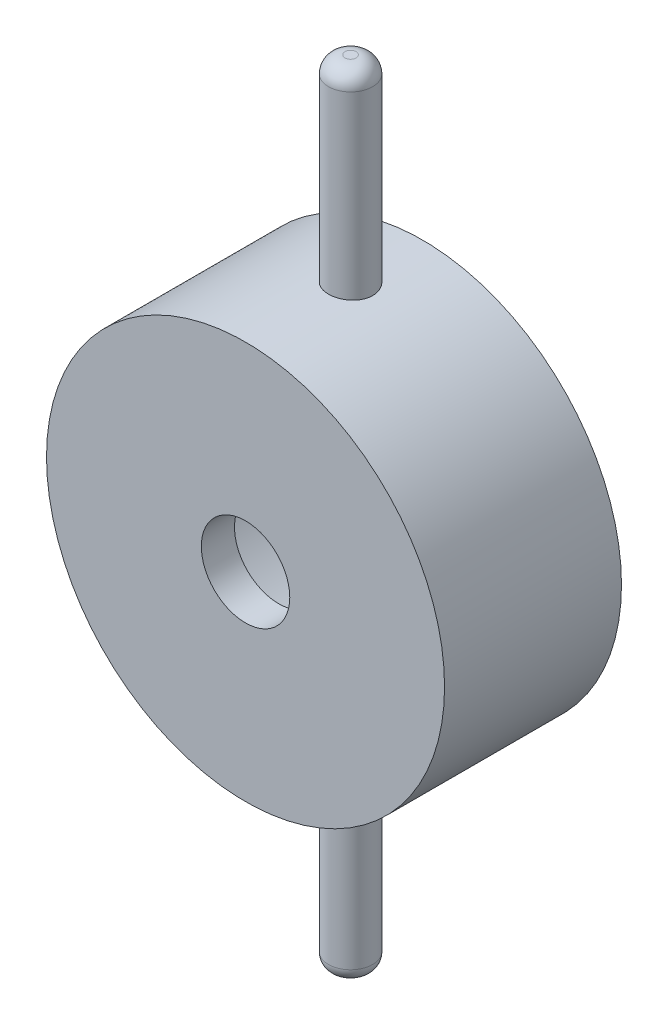
SolidWorks part; units mm, degrees
material "Plain Carbon Steel"
ref_plane "Front Plane" through (0, 0, 0) normal (0, 0, 1) x (1, 0, 0)
ref_plane "Top Plane" through (0, 0, 0) normal (0, 1, 0) x (1, 0, 0)
ref_plane "Right Plane" through (0, 0, 0) normal (1, 0, 0) x (0, 0, -1)
sketch "Hub Profile Sketch" plane through (0, 0, 0) normal (0, 0, 1) x (1, 0, 0)
  line L0 (0, 52.0937) -> (0, -51.5417) construction
  line L1 (70.2403, 0) -> (-66.3764, 0) construction
  circle A0 centre (0, 0) radius 36
  dimension "D1" = 72
extrude "Hub Ø72x32" add sketch "Hub Profile Sketch" along normal blind 32
sketch "Handle Pin Sketch Ø8" plane through (0, 0, 0) normal (0, 1, 0) x (1, 0, 0)
  line L0 (36, 0) -> (-36, 0) construction
  circle A0 centre (0, -13) radius 4
  dimension "D1" = 8
  dimension "D2" = 13
extrude "Handle Pin Ø8" add sketch "Handle Pin Sketch Ø8" along normal blind 36 from offset 35.5
fillet "Pin End Fillet R3" radius 3 1 edges at (0, 71.5, 17)
mirror "Handle Pin Mirror" about plane through (0, 0, 0) normal (0, 1, 0) of "Handle Pin Ø8"
sketch "Revolved Cut Sketch" plane through (0, 0, 0) normal (0, 1, 0) x (1, 0, 0)
  line L0 (0, 9.5355) -> (0, -35.1236) construction
  line L1 (0, -26) -> (-10, -26)
  line L2 (-10, -26) -> (-10, -28)
  line L3 (-10, -28) -> (-28, -28)
  line L4 (-28, -28) -> (-28, 0)
  line L5 (36, 0) -> (-36, 0) construction
  line L6 (-36, -32) -> (36, -32) construction
  line L7 (-28, 0) -> (0, 0)
  line L8 (0, 0) -> (0, -26)
  dimension "D1" = 10
  dimension "D2" = 2
  dimension "D3" = 6
  dimension "D4" = 28
revolve "Revolved Cut" cut sketch "Revolved Cut Sketch" angle 360 about L0
sketch "Face Recess Sketch Ø16" plane through (0, 0, 32) normal (0, 0, 1) x (1, 0, 0)
  circle A0 centre (0, 0) radius 8
  dimension "D1" = 16
extrude "Face Recess Ø16x6" cut sketch "Face Recess Sketch Ø16" against normal blind 6
fillet "Mirrored Pin Fillet R2.5" radius 2.5 1 edges at (0, -71.5, 17)
